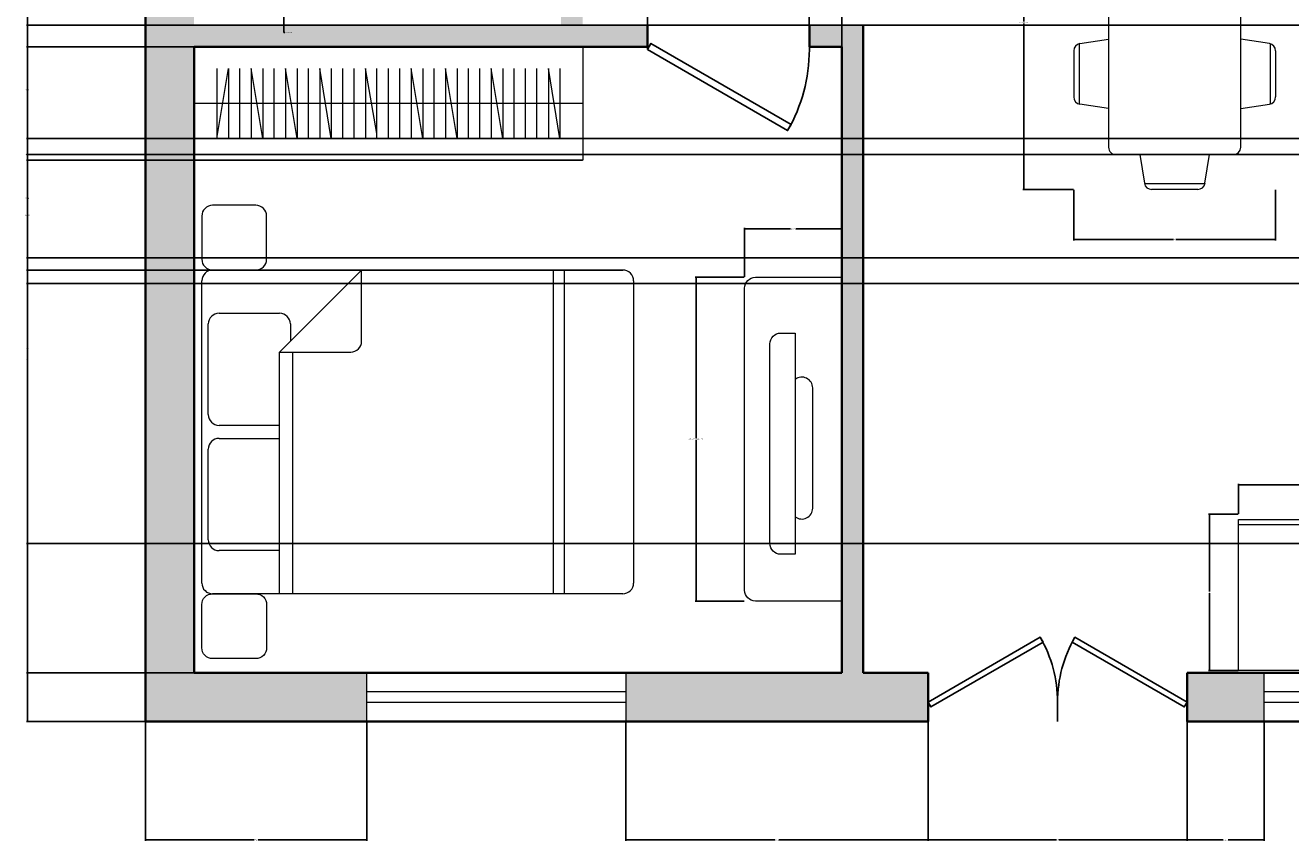
# Model space of a CAD drawing. Units: inches. Extents: x 2800 to 3283, y 1752 to 2114.
# Tile 1 of 6: x 2800 to 3035, y 1752 to 1903. Entities that reach past the tile are written whole.
import ezdxf

# ---------------------------------------------------------------- set-up
doc = ezdxf.new("R2010")
doc.units = ezdxf.units.IN
for name, color, linetype, lineweight in [('A-ANNO-DIMS', 2, 'Continuous', 18), ('A-DOOR', 3, 'Continuous', 25), ('A-EQPM', 8, 'Continuous', 18), ('A-FLOR-CASE', 8, 'Continuous', 18), ('A-FURN', 9, 'Continuous', 18), ('A-GLAZ', 4, 'Continuous', 18), ('A-WALL', 7, 'Continuous', 35)]:
    doc.layers.add(name, color=color, linetype=linetype, lineweight=lineweight)
doc.layers.add('A-WALL-PATT', color=18, linetype='Continuous', lineweight=13, true_color=0x000000)
doc.styles.get("Standard").update_dxf_attribs({"font": 'arial.ttf'})
doc.dimstyles.get("Standard").update_dxf_attribs({"dimtxt": 0.18, "dimasz": 0.18, "dimexe": 0.18, "dimexo": 0.0625, "dimgap": 0.09, "dimtad": 0, "dimtih": 1, "dimtoh": 1, "dimdec": 4, "dimzin": 0, "dimdsep": 46, "dimtxsty": 'Standard', "dimcen": 0.09, "dimadec": 0, "dimazin": 0, "dimtfac": 1, "dimtdec": 4, "dimtofl": 0, "dimtmove": 0, "dimatfit": 3, "dimfxl": 1, "dimtolj": 1, "dimtzin": 0, "dimarcsym": 0})

# ---------------------------------------------------------------- blocks, each defined once
blk = doc.blocks.new('Dining Set - 36 x 72 in.')
for p, q in [((-22.26, 25.81), (-23.48, 18)), ((-22.22, 26), (-5.78, 26)), ((-20.29, 27.5), (-7.71, 27.5)), ((-4.52, 18), (-5.74, 25.81)), ((5.74, 25.81), (4.52, 18)), ((5.78, 26), (22.22, 26)), ((7.71, 27.5), (20.29, 27.5)), ((23.48, 18), (22.26, 25.81)), ((34, 18), (-34, 18)), ((-36, 16), (-36, -16)), ((36, -16), (36, 16)), ((-44, 8.22), (-44, -8.22)), ((-43.81, 8.26), (-36, 9.48)), ((43.81, 8.26), (36, 9.48)), ((44, 8.22), (44, -8.22)), ((-45.5, 6.29), (-45.5, -6.29)), ((45.5, 6.29), (45.5, -6.29)), ((-36, -9.48), (-43.81, -8.26)), ((36, -9.48), (43.81, -8.26)), ((-34, -18), (34, -18)), ((-22.26, -25.81), (-23.48, -18)), ((-4.52, -18), (-5.74, -25.81)), ((5.74, -25.81), (4.52, -18)), ((23.48, -18), (22.26, -25.81)), ((-22.22, -26), (-5.78, -26)), ((-20.29, -27.5), (-7.71, -27.5)), ((5.78, -26), (22.22, -26)), ((7.71, -27.5), (20.29, -27.5))]:
    blk.add_line(p, q)
for centre, start, end in [((-20.29, 25.5), 90, 171.1198), ((-7.71, 25.5), 8.881, 90), ((7.71, 25.5), 90, 171.1198), ((20.29, 25.5), 8.881, 90), ((-34, 16), 90, 180), ((34, 16), 0, 90), ((-43.5, 6.29), 98.8806, 180), ((43.5, 6.29), 0, 81.1194), ((-43.5, -6.29), 180, 261.1194), ((43.5, -6.29), 278.8806, 0), ((-34, -16), 180, 270), ((34, -16), 270, 0), ((-20.29, -25.5), 188.8802, 270), ((-7.71, -25.5), 270, 351.1191), ((7.71, -25.5), 188.8802, 270), ((20.29, -25.5), 270, 351.1191)]:
    blk.add_arc(centre, 2, start, end)
blk = doc.blocks.new('Bed - Queen')
for p, q in [((2, 0), (58, 0)), ((0, -78), (0, -2)), ((10, -1.2), (26.8, -1.2)), ((33.2, -1.2), (50, -1.2)), ((60, -2), (60, -78)), ((8, -14.4), (8, -3.2)), ((28.8, -3.2), (28.8, -14.4)), ((31.2, -14.4), (31.2, -3.2)), ((52, -3.2), (52, -14.4)), ((0, -14.4), (44.8, -14.4)), ((60, -29.6), (44.8, -14.4)), ((44.8, -14.4), (44.8, -27.6)), ((50, -16.4), (46.8, -16.4)), ((44.8, -16.8), (0, -16.8)), ((46.8, -29.6), (60, -29.6)), ((0, -65.18), (60, -65.18)), ((0, -67.18), (60, -67.18)), ((58, -80), (2, -80))]:
    blk.add_line(p, q)
for centre, start, end in [((58, -2), 0, 90), ((2, -2), 90, 180), ((10, -3.2), 90, 180), ((26.8, -3.2), 0, 90), ((33.2, -3.2), 90, 180), ((50, -3.2), 0, 90), ((50, -14.4), 270, 0), ((46.8, -27.6), 180, 270), ((2, -78), 180, 270), ((58, -78), 270, 0)]:
    blk.add_arc(centre, 2, start, end)
blk = doc.blocks.new('Refrigerator-2 door - 36 in top')
for p, q in [((0, -26.999999), (36, -26.999999)), ((11, -27.999999), (11, -28.999999)), ((12, -26.999999), (12, -28.999999)), ((13, -28.999999), (13, -27.999999)), ((11, -28.999999), (13, -28.999999))]:
    blk.add_line(p, q)
blk.add_lwpolyline([(0, -27.999999), (0, 0), (36, 0), (36, -27.999999)], close=True)
blk = doc.blocks.new('*U12')
for p, q in [((0, 0), (0, -6)), ((40, 0), (40, -6))]:
    blk.add_line(p, q)
blk.add_lwpolyline([(0, 0), (34.64, 20), (35.52, 18.48), (0.87, -1.52)], close=True)
blk.add_arc((0, 0), 40, 0, 30)
blk = doc.blocks.new('*U13')
for p, q in [((0, 0), (0, 6)), ((40, 0), (40, 6))]:
    blk.add_line(p, q)
blk.add_lwpolyline([(0, 0), (34.64, -20), (35.52, -18.48), (0.87, 1.52)], close=True)
blk.add_arc((0, 0), 40, 330, 0)
blk = doc.blocks.new('WARDROBE-72')
for p, q in [((10.5, 72), (10.5, 0)), ((17, 63.53), (4, 63.53)), ((17, 61.41), (4, 61.41)), ((17, 59.29), (4, 59.29)), ((17, 52.94), (4, 52.94)), ((17, 50.82), (4, 50.82)), ((17, 44.47), (4, 44.47)), ((17, 38.12), (4, 38.12)), ((17, 36), (4, 36)), ((17, 33.88), (4, 33.88)), ((17, 29.65), (4, 29.65)), ((17, 27.53), (4, 27.53)), ((17, 21.18), (4, 21.18)), ((17, 14.82), (4, 14.82)), ((17, 8.47), (4, 8.47))]:
    blk.add_line(p, q)
for points in [[(0, 0), (0, 72), (21, 72), (21, 0), (0, 0), (21, 0)], [(4, 67.76), (17, 67.76), (4, 65.65), (17, 65.65)], [(4, 57.18), (17, 57.18), (4, 55.06), (17, 55.06)], [(4, 48.71), (17, 48.71), (4, 46.59), (17, 46.59)], [(4, 42.35), (17, 42.35), (4, 40.23), (17, 40.23)], [(16.02, 33.88), (4, 31.76), (17, 31.76)], [(4, 25.41), (17, 25.41), (4, 23.29), (17, 23.29)], [(4, 19.06), (17, 19.06), (4, 16.94), (17, 16.94)], [(4, 12.71), (17, 12.71), (4, 10.59), (17, 10.59)], [(4, 4.23), (17, 4.23), (4, 6.35), (17, 6.35)]]:
    blk.add_lwpolyline(points)
blk = doc.blocks.new('WIN-48')
for p, q in [((0, 5.5), (48, 5.5)), ((0, 3.5), (48, 3.5))]:
    blk.add_line(p, q)
for points in [[(0, 0), (0, 9)], [(48, 9), (48, 0)]]:
    blk.add_lwpolyline(points)
blk = doc.blocks.new('MEDIA-CONSOLE-60')
for points in [[(0, 60), (16, 60, -0.414214), (18, 58), (18, 2, -0.414214), (16, 0), (0, 0)], [(8.61, 51.33), (11.3, 51.33, -0.414214), (13.3, 49.33), (13.3, 12.33, -0.414214), (11.3, 10.33), (8.61, 10.33)]]:
    blk.add_lwpolyline(points, format="xyb", close=True)
blk.add_lwpolyline([(8.61, 15.1), (8.61, 47.68)])
blk.add_lwpolyline([(8.61, 44.37, 0.62446), (5.38, 42.79), (5.38, 20.5, 0.62446), (8.61, 18.92, 0.62446)], format="xyb")
blk = doc.blocks.new('NIGHTSTAND-12')
blk.add_lwpolyline([(2, 0), (10, 0, 0.414214), (12, 2), (12, 10, 0.414214), (10, 12), (2, 12, 0.414214), (0, 10), (0, 2, 0.414214)], format="xyb", close=True)
blk = doc.blocks.new('*D27')
at = {"layer": 'A-ANNO-DIMS', "color": 0, "lineweight": -2, "transparency": 16777216}
for p, q in [((2933.48, 1856.57), (2924.36, 1856.57)), ((2924.54, 1856.39), (2924.54, 1826.75)), ((2924.54, 1796.75), (2924.54, 1826.39)), ((2933.48, 1796.57), (2924.36, 1796.57))]:
    blk.add_line(p, q, dxfattribs=at)
at = {"layer": 'A-ANNO-DIMS', "color": 0, "transparency": 16777216}
for points in [[(2924.51, 1856.39), (2924.57, 1856.39), (2924.54, 1856.57)], [(2924.51, 1796.75), (2924.57, 1796.75), (2924.54, 1796.57)]]:
    blk.add_solid(points, dxfattribs=at)
at = {"layer": 'Defpoints', "color": 0, "transparency": 16777216}
for p in [(2933.54, 1856.57), (2924.54, 1796.57), (2933.54, 1796.57)]:
    blk.add_point(p, dxfattribs=at)
at = {"layer": 'A-ANNO-DIMS', "color": 0, "transparency": 16777216, "insert": (2924.54, 1826.57), "char_height": 0.18, "attachment_point": 5}
blk.add_mtext('\\A1;MEDIA CONSOLE 60 TYP.', dxfattribs=at)
blk = doc.blocks.new('*D28')
at = {"layer": 'A-ANNO-DIMS', "color": 0, "lineweight": -2, "transparency": 16777216}
for p, q in [((2933.54, 1856.63), (2933.54, 1865.75)), ((2933.72, 1865.57), (2942.02, 1865.57)), ((2951.36, 1865.57), (2943.06, 1865.57)), ((2951.54, 1856.63), (2951.54, 1865.75))]:
    blk.add_line(p, q, dxfattribs=at)
at = {"layer": 'A-ANNO-DIMS', "color": 0, "transparency": 16777216}
for points in [[(2933.72, 1865.6), (2933.72, 1865.54), (2933.54, 1865.57)], [(2951.36, 1865.6), (2951.36, 1865.54), (2951.54, 1865.57)]]:
    blk.add_solid(points, dxfattribs=at)
at = {"layer": 'Defpoints', "color": 0, "transparency": 16777216}
for p in [(2933.54, 1865.57), (2933.54, 1856.57), (2951.54, 1856.57)]:
    blk.add_point(p, dxfattribs=at)
at = {"layer": 'A-ANNO-DIMS', "color": 0, "transparency": 16777216, "insert": (2942.54, 1865.57), "char_height": 0.18, "attachment_point": 5}
blk.add_mtext('\\A1;18 TYP.', dxfattribs=at)
blk = doc.blocks.new('*D35')
at = {"layer": 'A-ANNO-DIMS', "color": 0, "lineweight": -2, "transparency": 16777216}
for p, q in [((2994.48, 1934.72), (2985.08, 1934.72)), ((2985.26, 1934.54), (2985.26, 1903.97)), ((2985.26, 1873.03), (2985.26, 1903.6)), ((2994.48, 1872.85), (2985.08, 1872.85))]:
    blk.add_line(p, q, dxfattribs=at)
at = {"layer": 'A-ANNO-DIMS', "color": 0, "transparency": 16777216}
for points in [[(2985.23, 1934.54), (2985.29, 1934.54), (2985.26, 1934.72)], [(2985.23, 1873.03), (2985.29, 1873.03), (2985.26, 1872.85)]]:
    blk.add_solid(points, dxfattribs=at)
at = {"layer": 'Defpoints', "color": 0, "transparency": 16777216}
for p in [(2994.54, 1934.72), (2985.26, 1872.85), (2994.54, 1872.85)]:
    blk.add_point(p, dxfattribs=at)
at = {"layer": 'A-ANNO-DIMS', "color": 0, "transparency": 16777216, "insert": (2985.26, 1903.79), "char_height": 0.18, "attachment_point": 5}
blk.add_mtext('\\A1;DINING SET 62', dxfattribs=at)
blk = doc.blocks.new('*D36')
at = {"layer": 'A-ANNO-DIMS', "color": 0, "lineweight": -2, "transparency": 16777216}
for p, q in [((2994.54, 1872.79), (2994.54, 1863.39)), ((3031.94, 1872.79), (3031.94, 1863.39)), ((2994.72, 1863.57), (3013.02, 1863.57)), ((3031.76, 1863.57), (3013.46, 1863.57))]:
    blk.add_line(p, q, dxfattribs=at)
at = {"layer": 'A-ANNO-DIMS', "color": 0, "transparency": 16777216}
for points in [[(2994.72, 1863.6), (2994.72, 1863.54), (2994.54, 1863.57)], [(3031.76, 1863.6), (3031.76, 1863.54), (3031.94, 1863.57)]]:
    blk.add_solid(points, dxfattribs=at)
at = {"layer": 'Defpoints', "color": 0, "transparency": 16777216}
for p in [(2994.54, 1872.85), (3031.94, 1872.85), (3031.94, 1863.57)]:
    blk.add_point(p, dxfattribs=at)
at = {"layer": 'A-ANNO-DIMS', "color": 0, "transparency": 16777216, "insert": (3013.24, 1863.57), "char_height": 0.18, "attachment_point": 5}
blk.add_mtext('\\A1;37', dxfattribs=at)
blk = doc.blocks.new('*D41')
at = {"layer": 'A-ANNO-DIMS', "color": 0, "lineweight": -2, "transparency": 16777216}
for p, q in [((3025.08, 1812.76), (3025.08, 1818.28)), ((3025.26, 1818.1), (3041.83, 1818.1)), ((3060.9, 1818.1), (3044.33, 1818.1)), ((3061.08, 1812.76), (3061.08, 1818.28))]:
    blk.add_line(p, q, dxfattribs=at)
at = {"layer": 'A-ANNO-DIMS', "color": 0, "transparency": 16777216}
for points in [[(3025.26, 1818.13), (3025.26, 1818.07), (3025.08, 1818.1)], [(3060.9, 1818.13), (3060.9, 1818.07), (3061.08, 1818.1)]]:
    blk.add_solid(points, dxfattribs=at)
at = {"layer": 'Defpoints', "color": 0, "transparency": 16777216}
for p in [(3025.08, 1818.1), (3025.08, 1812.7), (3061.08, 1812.7)]:
    blk.add_point(p, dxfattribs=at)
at = {"layer": 'A-ANNO-DIMS', "color": 0, "transparency": 16777216, "insert": (3043.08, 1818.1), "char_height": 0.18, "attachment_point": 5}
blk.add_mtext('\\A1;REFRIGERATOR 36', dxfattribs=at)
blk = doc.blocks.new('*D42')
at = {"layer": 'A-ANNO-DIMS', "color": 0, "lineweight": -2, "transparency": 16777216}
for p, q in [((3025.02, 1812.7), (3019.5, 1812.7)), ((3019.68, 1812.52), (3019.68, 1798.38)), ((3019.68, 1783.88), (3019.68, 1798.02)), ((3025.02, 1783.7), (3019.5, 1783.7))]:
    blk.add_line(p, q, dxfattribs=at)
at = {"layer": 'A-ANNO-DIMS', "color": 0, "transparency": 16777216}
for points in [[(3019.65, 1812.52), (3019.71, 1812.52), (3019.68, 1812.7)], [(3019.65, 1783.88), (3019.71, 1783.88), (3019.68, 1783.7)]]:
    blk.add_solid(points, dxfattribs=at)
at = {"layer": 'Defpoints', "color": 0, "transparency": 16777216}
for p in [(3025.08, 1812.7), (3019.68, 1783.7), (3025.08, 1783.7)]:
    blk.add_point(p, dxfattribs=at)
at = {"layer": 'A-ANNO-DIMS', "color": 0, "transparency": 16777216, "insert": (3019.68, 1798.2), "char_height": 0.18, "attachment_point": 5}
blk.add_mtext('\\A1;29', dxfattribs=at)
blk = doc.blocks.new('*D44')
at = {"layer": 'A-ANNO-DIMS', "color": 0, "lineweight": -2, "transparency": 16777216}
for p, q in [((2822.48, 2092.27), (2800.45, 2092.27)), ((2800.63, 2092.09), (2800.63, 1933.45)), ((2800.63, 1774.45), (2800.63, 1933.09)), ((2822.48, 1774.27), (2800.45, 1774.27))]:
    blk.add_line(p, q, dxfattribs=at)
at = {"layer": 'A-ANNO-DIMS', "color": 0, "transparency": 16777216}
for points in [[(2800.6, 2092.09), (2800.66, 2092.09), (2800.63, 2092.27)], [(2800.6, 1774.45), (2800.66, 1774.45), (2800.63, 1774.27)]]:
    blk.add_solid(points, dxfattribs=at)
at = {"layer": 'Defpoints', "color": 0, "transparency": 16777216}
for p in [(2800.63, 2092.27), (2822.54, 2092.27), (2822.54, 1774.27)]:
    blk.add_point(p, dxfattribs=at)
at = {"layer": 'A-ANNO-DIMS', "color": 0, "transparency": 16777216, "insert": (2800.63, 1933.27), "char_height": 0.18, "attachment_point": 5}
blk.add_mtext('\\A1;318', dxfattribs=at)
blk = doc.blocks.new('*D51')
at = {"layer": 'A-ANNO-DIMS', "color": 0, "lineweight": -2, "transparency": 16777216}
for p, q in [((2831.48, 1899.27), (2800.45, 1899.27)), ((2800.63, 1899.09), (2800.63, 1841.45)), ((2800.63, 1783.45), (2800.63, 1841.09)), ((2831.48, 1783.27), (2800.45, 1783.27))]:
    blk.add_line(p, q, dxfattribs=at)
at = {"layer": 'A-ANNO-DIMS', "color": 0, "transparency": 16777216}
for points in [[(2800.6, 1899.09), (2800.66, 1899.09), (2800.63, 1899.27)], [(2800.6, 1783.45), (2800.66, 1783.45), (2800.63, 1783.27)]]:
    blk.add_solid(points, dxfattribs=at)
at = {"layer": 'Defpoints', "color": 0, "transparency": 16777216}
for p in [(2800.63, 1899.27), (2831.54, 1899.27), (2831.54, 1783.27)]:
    blk.add_point(p, dxfattribs=at)
at = {"layer": 'A-ANNO-DIMS', "color": 0, "transparency": 16777216, "insert": (2800.63, 1841.27), "char_height": 0.18, "attachment_point": 5}
blk.add_mtext('\\A1;116', dxfattribs=at)
blk = doc.blocks.new('*D59')
at = {"layer": 'A-ANNO-DIMS', "color": 0, "lineweight": -2, "transparency": 16777216}
for p, q in [((2822.54, 1774.21), (2822.54, 1752.17)), ((2863.53, 1774.21), (2863.53, 1752.17)), ((2822.72, 1752.35), (2842.64, 1752.35)), ((2863.35, 1752.35), (2843.43, 1752.35))]:
    blk.add_line(p, q, dxfattribs=at)
at = {"layer": 'A-ANNO-DIMS', "color": 0, "transparency": 16777216}
for points in [[(2822.72, 1752.38), (2822.72, 1752.32), (2822.54, 1752.35)], [(2863.35, 1752.38), (2863.35, 1752.32), (2863.53, 1752.35)]]:
    blk.add_solid(points, dxfattribs=at)
at = {"layer": 'Defpoints', "color": 0, "transparency": 16777216}
for p in [(2822.54, 1774.27), (2863.53, 1774.27), (2863.53, 1752.35)]:
    blk.add_point(p, dxfattribs=at)
at = {"layer": 'A-ANNO-DIMS', "color": 0, "transparency": 16777216, "insert": (2843.04, 1752.35), "char_height": 0.18, "attachment_point": 5}
blk.add_mtext('\\A1;40.99', dxfattribs=at)
blk = doc.blocks.new('*D60')
at = {"layer": 'A-ANNO-DIMS', "color": 0, "lineweight": -2, "transparency": 16777216}
for p, q in [((2911.53, 1774.21), (2911.53, 1752.17)), ((2967.54, 1774.21), (2967.54, 1752.17)), ((2911.71, 1752.35), (2939.16, 1752.35)), ((2967.36, 1752.35), (2939.91, 1752.35))]:
    blk.add_line(p, q, dxfattribs=at)
at = {"layer": 'A-ANNO-DIMS', "color": 0, "transparency": 16777216}
for points in [[(2911.71, 1752.38), (2911.71, 1752.32), (2911.53, 1752.35)], [(2967.36, 1752.38), (2967.36, 1752.32), (2967.54, 1752.35)]]:
    blk.add_solid(points, dxfattribs=at)
at = {"layer": 'Defpoints', "color": 0, "transparency": 16777216}
for p in [(2911.53, 1774.27), (2967.54, 1774.27), (2967.54, 1752.35)]:
    blk.add_point(p, dxfattribs=at)
at = {"layer": 'A-ANNO-DIMS', "color": 0, "transparency": 16777216, "insert": (2939.54, 1752.35), "char_height": 0.18, "attachment_point": 5}
blk.add_mtext('\\A1;56.01', dxfattribs=at)
blk = doc.blocks.new('*D61')
at = {"layer": 'A-ANNO-DIMS', "color": 0, "lineweight": -2, "transparency": 16777216}
for p, q in [((2967.54, 1774.21), (2967.54, 1752.17)), ((3015.54, 1774.21), (3015.54, 1752.17)), ((2967.72, 1752.35), (2991.32, 1752.35)), ((3015.36, 1752.35), (2991.77, 1752.35))]:
    blk.add_line(p, q, dxfattribs=at)
at = {"layer": 'A-ANNO-DIMS', "color": 0, "transparency": 16777216}
for points in [[(2967.72, 1752.38), (2967.72, 1752.32), (2967.54, 1752.35)], [(3015.36, 1752.38), (3015.36, 1752.32), (3015.54, 1752.35)]]:
    blk.add_solid(points, dxfattribs=at)
at = {"layer": 'Defpoints', "color": 0, "transparency": 16777216}
for p in [(2967.54, 1774.27), (3015.54, 1774.27), (3015.54, 1752.35)]:
    blk.add_point(p, dxfattribs=at)
at = {"layer": 'A-ANNO-DIMS', "color": 0, "transparency": 16777216, "insert": (2991.54, 1752.35), "char_height": 0.18, "attachment_point": 5}
blk.add_mtext('\\A1;48', dxfattribs=at)
blk = doc.blocks.new('*D62')
at = {"layer": 'A-ANNO-DIMS', "color": 0, "lineweight": -2, "transparency": 16777216}
for p, q in [((3015.54, 1774.21), (3015.54, 1752.17)), ((3029.8, 1774.21), (3029.8, 1752.17)), ((3015.72, 1752.35), (3022.22, 1752.35)), ((3029.62, 1752.35), (3023.13, 1752.35))]:
    blk.add_line(p, q, dxfattribs=at)
at = {"layer": 'A-ANNO-DIMS', "color": 0, "transparency": 16777216}
for points in [[(3015.72, 1752.38), (3015.72, 1752.32), (3015.54, 1752.35)], [(3029.62, 1752.38), (3029.62, 1752.32), (3029.8, 1752.35)]]:
    blk.add_solid(points, dxfattribs=at)
at = {"layer": 'Defpoints', "color": 0, "transparency": 16777216}
for p in [(3015.54, 1774.27), (3029.8, 1774.27), (3029.8, 1752.35)]:
    blk.add_point(p, dxfattribs=at)
at = {"layer": 'A-ANNO-DIMS', "color": 0, "transparency": 16777216, "insert": (3022.67, 1752.35), "char_height": 0.18, "attachment_point": 5}
blk.add_mtext('\\A1;14.258', dxfattribs=at)
blk = doc.blocks.new('*D66')
at = {"layer": 'A-ANNO-DIMS', "color": 0, "lineweight": -2, "transparency": 16777216}
for p, q in [((2915.54, 1899.33), (2915.54, 2114.36)), ((2915.72, 2114.18), (2930.32, 2114.18)), ((2945.36, 2114.18), (2930.76, 2114.18)), ((2945.54, 1899.33), (2945.54, 2114.36))]:
    blk.add_line(p, q, dxfattribs=at)
at = {"layer": 'A-ANNO-DIMS', "color": 0, "transparency": 16777216}
for points in [[(2915.72, 2114.21), (2915.72, 2114.15), (2915.54, 2114.18)], [(2945.36, 2114.21), (2945.36, 2114.15), (2945.54, 2114.18)]]:
    blk.add_solid(points, dxfattribs=at)
at = {"layer": 'Defpoints', "color": 0, "transparency": 16777216}
for p in [(2945.54, 2114.18), (2915.54, 1899.27), (2945.54, 1899.27)]:
    blk.add_point(p, dxfattribs=at)
at = {"layer": 'A-ANNO-DIMS', "color": 0, "transparency": 16777216, "insert": (2930.54, 2114.18), "char_height": 0.18, "attachment_point": 5}
blk.add_mtext('\\A1;30', dxfattribs=at)
blk = doc.blocks.new('*D67')
at = {"layer": 'A-ANNO-DIMS', "color": 0, "lineweight": -2, "transparency": 16777216}
for p, q in [((2945.54, 1899.33), (2945.54, 2114.36)), ((2945.72, 2114.18), (2948.39, 2114.18)), ((2951.36, 2114.18), (2948.69, 2114.18)), ((2951.54, 1899.33), (2951.54, 2114.36))]:
    blk.add_line(p, q, dxfattribs=at)
at = {"layer": 'A-ANNO-DIMS', "color": 0, "transparency": 16777216}
for points in [[(2945.72, 2114.21), (2945.72, 2114.15), (2945.54, 2114.18)], [(2951.36, 2114.21), (2951.36, 2114.15), (2951.54, 2114.18)]]:
    blk.add_solid(points, dxfattribs=at)
at = {"layer": 'Defpoints', "color": 0, "transparency": 16777216}
for p in [(2951.54, 2114.18), (2945.54, 1899.27), (2951.54, 1899.27)]:
    blk.add_point(p, dxfattribs=at)
at = {"layer": 'A-ANNO-DIMS', "color": 0, "transparency": 16777216, "insert": (2948.54, 2114.18), "char_height": 0.18, "attachment_point": 5}
blk.add_mtext('\\A1;6', dxfattribs=at)
blk = doc.blocks.new('*D71')
at = {"layer": 'A-ANNO-DIMS', "color": 0, "lineweight": -2, "transparency": 16777216}
for p, q in [((3037.48, 1903.27), (2800.45, 1903.27)), ((2800.63, 1903.09), (2800.63, 1879.54)), ((2800.63, 1855.63), (2800.63, 1879.18)), ((3037.48, 1855.45), (2800.45, 1855.45))]:
    blk.add_line(p, q, dxfattribs=at)
at = {"layer": 'A-ANNO-DIMS', "color": 0, "transparency": 16777216}
for points in [[(2800.6, 1903.09), (2800.66, 1903.09), (2800.63, 1903.27)], [(2800.6, 1855.63), (2800.66, 1855.63), (2800.63, 1855.45)]]:
    blk.add_solid(points, dxfattribs=at)
at = {"layer": 'Defpoints', "color": 0, "transparency": 16777216}
for p in [(2800.63, 1903.27), (3037.54, 1903.27), (3037.54, 1855.45)]:
    blk.add_point(p, dxfattribs=at)
at = {"layer": 'A-ANNO-DIMS', "color": 0, "transparency": 16777216, "insert": (2800.63, 1879.36), "char_height": 0.18, "attachment_point": 5}
blk.add_mtext('\\A1;47.82', dxfattribs=at)
blk = doc.blocks.new('*D73')
at = {"layer": 'A-ANNO-DIMS', "color": 0, "lineweight": -2, "transparency": 16777216}
for p, q in [((3103.48, 1879.34), (2800.45, 1879.34)), ((2800.63, 1879.16), (2800.63, 1843.49)), ((2800.63, 1807.45), (2800.63, 1843.12)), ((3103.48, 1807.27), (2800.45, 1807.27))]:
    blk.add_line(p, q, dxfattribs=at)
at = {"layer": 'A-ANNO-DIMS', "color": 0, "transparency": 16777216}
for points in [[(2800.6, 1879.16), (2800.66, 1879.16), (2800.63, 1879.34)], [(2800.6, 1807.45), (2800.66, 1807.45), (2800.63, 1807.27)]]:
    blk.add_solid(points, dxfattribs=at)
at = {"layer": 'Defpoints', "color": 0, "transparency": 16777216}
for p in [(2800.63, 1879.34), (3103.54, 1879.34), (3103.54, 1807.27)]:
    blk.add_point(p, dxfattribs=at)
at = {"layer": 'A-ANNO-DIMS', "color": 0, "transparency": 16777216, "insert": (2800.63, 1843.31), "char_height": 0.18, "attachment_point": 5}
blk.add_mtext('\\A1;72.07', dxfattribs=at)
blk = doc.blocks.new('*D76')
at = {"layer": 'A-ANNO-DIMS', "color": 0, "lineweight": -2, "transparency": 16777216}
for p, q in [((3095.48, 1903.27), (2800.45, 1903.27)), ((2800.63, 1903.09), (2800.63, 1891.49)), ((2800.63, 1879.52), (2800.63, 1891.12)), ((3103.48, 1879.34), (2800.45, 1879.34))]:
    blk.add_line(p, q, dxfattribs=at)
at = {"layer": 'A-ANNO-DIMS', "color": 0, "transparency": 16777216}
for points in [[(2800.6, 1903.09), (2800.66, 1903.09), (2800.63, 1903.27)], [(2800.6, 1879.52), (2800.66, 1879.52), (2800.63, 1879.34)]]:
    blk.add_solid(points, dxfattribs=at)
at = {"layer": 'Defpoints', "color": 0, "transparency": 16777216}
for p in [(3095.54, 1903.27), (2800.63, 1879.34), (3103.54, 1879.34)]:
    blk.add_point(p, dxfattribs=at)
at = {"layer": 'A-ANNO-DIMS', "color": 0, "transparency": 16777216, "insert": (2800.63, 1891.31), "char_height": 0.18, "attachment_point": 5}
blk.add_mtext('\\A1;23.93', dxfattribs=at)
blk = doc.blocks.new('*D83')
at = {"layer": 'A-ANNO-DIMS', "color": 0, "lineweight": -2, "transparency": 16777216}
for p, q in [((2903.48, 1878.27), (2800.45, 1878.27)), ((2800.63, 1878.09), (2800.63, 1868.28)), ((2800.63, 1858.1), (2800.63, 1867.91)), ((2910.9, 1857.92), (2800.45, 1857.92))]:
    blk.add_line(p, q, dxfattribs=at)
at = {"layer": 'A-ANNO-DIMS', "color": 0, "transparency": 16777216}
for points in [[(2800.6, 1878.09), (2800.66, 1878.09), (2800.63, 1878.27)], [(2800.6, 1858.1), (2800.66, 1858.1), (2800.63, 1857.92)]]:
    blk.add_solid(points, dxfattribs=at)
at = {"layer": 'Defpoints', "color": 0, "transparency": 16777216}
for p in [(2903.54, 1878.27), (2800.63, 1857.92), (2910.97, 1857.92)]:
    blk.add_point(p, dxfattribs=at)
at = {"layer": 'A-ANNO-DIMS', "color": 0, "transparency": 16777216, "insert": (2800.63, 1868.1), "char_height": 0.18, "attachment_point": 5}
blk.add_mtext('\\A1;20.348', dxfattribs=at)
blk = doc.blocks.new('*D84')
at = {"layer": 'A-ANNO-DIMS', "color": 0, "lineweight": -2, "transparency": 16777216}
for p, q in [((3179.48, 1882.27), (2800.45, 1882.27)), ((2800.63, 1882.09), (2800.63, 1871.42)), ((2800.63, 1860.39), (2800.63, 1871.06)), ((3172.07, 1860.21), (2800.45, 1860.21))]:
    blk.add_line(p, q, dxfattribs=at)
at = {"layer": 'A-ANNO-DIMS', "color": 0, "transparency": 16777216}
for points in [[(2800.6, 1882.09), (2800.66, 1882.09), (2800.63, 1882.27)], [(2800.6, 1860.39), (2800.66, 1860.39), (2800.63, 1860.21)]]:
    blk.add_solid(points, dxfattribs=at)
at = {"layer": 'Defpoints', "color": 0, "transparency": 16777216}
for p in [(3179.54, 1882.27), (2800.63, 1860.21), (3172.14, 1860.21)]:
    blk.add_point(p, dxfattribs=at)
at = {"layer": 'A-ANNO-DIMS', "color": 0, "transparency": 16777216, "insert": (2800.63, 1871.24), "char_height": 0.18, "attachment_point": 5}
blk.add_mtext('\\A1;22.06', dxfattribs=at)
blk = doc.blocks.new('*D87')
at = {"layer": 'A-ANNO-DIMS', "color": 0, "lineweight": -2, "transparency": 16777216}
for p, q in [((2848.06, 1921.79), (2848.24, 1921.79)), ((2848.15, 1921.7), (2848.15, 1921.88)), ((2848.15, 1901.96), (2848.15, 1909.22)), ((2848.33, 1901.96), (2848.15, 1901.96))]:
    blk.add_line(p, q, dxfattribs=at)
at = {"layer": 'A-ANNO-DIMS', "color": 0, "transparency": 16777216}
blk.add_solid([(2848.18, 1909.22), (2848.12, 1909.22), (2848.15, 1909.4)], dxfattribs=at)
at = {"layer": 'Defpoints', "color": 0, "transparency": 16777216}
for p in [(2848.15, 1921.79), (2848.15, 1909.4)]:
    blk.add_point(p, dxfattribs=at)
at = {"layer": 'A-ANNO-DIMS', "color": 0, "transparency": 16777216, "insert": (2849.06, 1901.96), "char_height": 0.18, "attachment_point": 5}
blk.add_mtext('\\A1;2X R12.391', dxfattribs=at)

msp = doc.modelspace()

# ---------------------------------------------------------------- hatches: boundary and pattern name
at = {"layer": 'A-WALL-PATT'}
h = msp.add_hatch(color=256, dxfattribs=at)
h.dxf.hatch_style = 1
h.paths.add_polyline_path([(2863.5307, 1783.2695), (2831.5432, 1783.2695), (2831.5432, 1899.2695), (2903.5432, 1899.2695), (2915.5432, 1899.2695), (2915.5432, 1903.2695), (2903.5432, 1903.2695), (2903.5432, 1933.2695), (2899.5432, 1933.2695), (2899.5432, 1903.2695), (2831.5432, 1903.2695), (2831.5432, 1922.3547), (2822.5432, 1922.3547), (2822.5432, 1774.2695), (2863.5307, 1774.2695)])
h = msp.add_hatch(color=256, dxfattribs=at)
h.dxf.hatch_style = 1
h.paths.add_polyline_path([(2967.5432, 1783.2695), (2955.5432, 1783.2695), (2955.5432, 1903.2695), (2945.5432, 1903.2695), (2945.5432, 1899.2695), (2951.5432, 1899.2695), (2951.5432, 1783.2695), (2911.5307, 1783.2695), (2911.5307, 1774.2695), (2967.5432, 1774.2695)])
h = msp.add_hatch(color=256, dxfattribs=at)
h.dxf.hatch_style = 1
h.paths.add_polyline_path([(3029.8011, 1783.2695), (3015.5432, 1783.2695), (3015.5432, 1774.2695), (3029.8011, 1774.2695)])

# ---------------------------------------------------------------- linework, layer by layer
at = {"layer": 'A-WALL'}
for p, q in [((2915.5432, 1899.2695), (2915.5432, 1903.2695)), ((2945.5432, 1899.2695), (2945.5432, 1903.2695)), ((2955.5432, 1783.2695), (2955.5432, 1903.2695)), ((2831.5432, 1783.2695), (2831.5432, 1899.2695)), ((2915.5432, 1899.2695), (2831.5432, 1899.2695)), ((2951.5432, 1899.2695), (2945.5432, 1899.2695)), ((2951.5432, 1783.2695), (2951.5432, 1899.2695)), ((2951.5432, 1783.2695), (2831.5432, 1783.2695)), ((2967.5432, 1783.2695), (2955.5432, 1783.2695)), ((2967.5432, 1783.2695), (2967.5432, 1774.2695)), ((3127.5432, 1783.2695), (3015.5432, 1783.2695)), ((3015.5432, 1783.2695), (3015.5432, 1774.2695))]:
    msp.add_line(p, q, dxfattribs=at)
msp.add_lwpolyline([(2967.5432, 1774.2695), (2822.5432, 1774.2695), (2822.5432, 2092.2695), (3260.5432, 2092.2695), (3260.5432, 1774.2695), (3015.5432, 1774.2695)], dxfattribs=at)

# ---------------------------------------------------------------- block references
at = {"layer": 'A-DOOR'}
for name, p, xscale, yscale, zscale in [('*U13', (2915.5432, 1898.7695), 0.75, 0.75, 0.75), ('*U12', (2967.5432, 1777.8695), 0.6, 0.6, 0.6), ('*U12', (3015.5432, 1777.8695), -0.6, 0.6, 0.6)]:
    msp.add_blockref(name, p, dxfattribs=dict(at, xscale=xscale, yscale=yscale, zscale=zscale))
at = {"layer": 'A-EQPM', "rotation": 180}
msp.add_blockref('Refrigerator-2 door - 36 in top', (3061.0792, 1783.7005), dxfattribs=at)
at = {"layer": 'A-FLOR-CASE', "rotation": 270}
msp.add_blockref('WARDROBE-72', (2831.5437, 1899.2697), dxfattribs=at)
at = {"layer": 'A-FURN', "xscale": 0.6798973634336658, "yscale": 0.6798973634336658, "zscale": 0.6798973634336658, "rotation": 270}
msp.add_blockref('Dining Set - 36 x 72 in.', (3013.2412, 1903.787), dxfattribs=at)
at = {"layer": 'A-FURN'}
msp.add_blockref('NIGHTSTAND-12', (2832.967, 1857.922), dxfattribs=at)
for name, p, rotation in [('Bed - Queen', (2832.9674, 1797.9218), 89.99999999999999), ('MEDIA-CONSOLE-60', (2951.5433, 1856.5689), 180)]:
    msp.add_blockref(name, p, dxfattribs=dict(at, rotation=rotation))
at = {"layer": 'A-FURN', "extrusion": (0, 0, -1), "zscale": -1, "rotation": 180}
msp.add_blockref('NIGHTSTAND-12', (-2832.967, 1797.9216), dxfattribs=at)
at = {"layer": 'A-GLAZ', "rotation": 180}
for p in [(2911.5306, 1783.269), (3077.801, 1783.269)]:
    msp.add_blockref('WIN-48', p, dxfattribs=at)

# ---------------------------------------------------------------- dimensions: what is measured, and where the dimension line sits
at = {"layer": 'A-ANNO-DIMS'}
for base, p1, p2, override, picture, middle in [((2945.5432, 2114.1845), (2915.5432, 1899.2695), (2945.5432, 1899.2695), {"dimdec": 0, "dimlfac": 1, "dimrnd": 0, "dimzin": 0, "dimdsep": 46, "dimlunit": 2}, '*D66', (2930.5432, 2114.1845)), ((2951.5432, 2114.1845), (2945.5432, 1899.2695), (2951.5432, 1899.2695), {"dimdec": 0, "dimlfac": 1, "dimrnd": 0, "dimzin": 0, "dimdsep": 46, "dimlunit": 2}, '*D67', (2948.5432, 2114.1845)), ((3031.9384, 1863.5711), (2994.5441, 1872.8517), (3031.9384, 1872.8517), {"dimdec": 0, "dimlfac": 1, "dimrnd": 0, "dimzin": 0, "dimdsep": 46, "dimlunit": 2}, '*D36', (3013.2412, 1863.5711)), ((2863.5307, 1752.3545), (2822.5432, 1774.2695), (2863.5307, 1774.2695), {"dimdec": 2, "dimlfac": 1, "dimrnd": 0, "dimzin": 0, "dimdsep": 46, "dimlunit": 2}, '*D59', (2843.037, 1752.3545)), ((2967.5432, 1752.3545), (2911.5307, 1774.2695), (2967.5432, 1774.2695), {"dimdec": 2, "dimlfac": 1, "dimrnd": 0, "dimzin": 0, "dimdsep": 46, "dimlunit": 2}, '*D60', (2939.537, 1752.3545)), ((3015.5432, 1752.3545), (2967.5432, 1774.2695), (3015.5432, 1774.2695), {"dimdec": 0, "dimlfac": 1, "dimrnd": 0, "dimzin": 0, "dimdsep": 46, "dimlunit": 2}, '*D61', (2991.5432, 1752.3545)), ((3029.8011, 1752.3545), (3015.5432, 1774.2695), (3029.8011, 1774.2695), {"dimdec": 3, "dimlfac": 1, "dimrnd": 0, "dimzin": 0, "dimdsep": 46, "dimlunit": 2}, '*D62', (3022.6722, 1752.3545))]:
    dim = msp.add_linear_dim(base=base, p1=p1, p2=p2, dimstyle='Standard', override=override, dxfattribs=at)
    dim.commit()
    dim.dimension.update_dxf_attribs({"geometry": picture, "text_midpoint": middle})
for base, p1, p2, angle, override, picture, middle in [((2800.6282, 2092.2695), (2822.5432, 1774.2695), (2822.5432, 2092.2695), 90, {"dimdec": 0, "dimlfac": 1, "dimrnd": 0, "dimzin": 0, "dimdsep": 46, "dimlunit": 2}, '*D44', (2800.6282, 1933.2695)), ((2800.6282, 1903.2695), (3037.5432, 1855.4517), (3037.5432, 1903.2695), 90, {"dimdec": 2, "dimlfac": 1, "dimrnd": 0, "dimzin": 0, "dimdsep": 46, "dimlunit": 2}, '*D71', (2800.6282, 1879.3606)), ((2800.6282, 1879.3408), (3095.5432, 1903.2695), (3103.5432, 1879.3408), 90, {"dimdec": 2, "dimlfac": 1, "dimrnd": 0, "dimzin": 0, "dimdsep": 46, "dimlunit": 2}, '*D76', (2800.6282, 1891.3052)), ((2800.6282, 1899.2695), (2831.5432, 1783.2695), (2831.5432, 1899.2695), 90, {"dimdec": 0, "dimlfac": 1, "dimrnd": 0, "dimzin": 0, "dimdsep": 46, "dimlunit": 2}, '*D51', (2800.6282, 1841.2695)), ((2800.6282, 1860.2087), (3179.5432, 1882.2695), (3172.1372, 1860.2087), 90, {"dimdec": 2, "dimlfac": 1, "dimrnd": 0, "dimzin": 0, "dimdsep": 46, "dimlunit": 2}, '*D84', (2800.6282, 1871.2391)), ((2800.6282, 1857.9218), (2903.5432, 1878.2695), (2910.9675, 1857.9218), 90, {"dimdec": 3, "dimlfac": 1, "dimrnd": 0, "dimzin": 0, "dimdsep": 46, "dimlunit": 2}, '*D83', (2800.6282, 1868.0956)), ((2800.6282, 1879.3408), (3103.5432, 1807.2695), (3103.5432, 1879.3408), 90, {"dimdec": 2, "dimlfac": 1, "dimrnd": 0, "dimzin": 0, "dimdsep": 46, "dimlunit": 2}, '*D73', (2800.6282, 1843.3052)), ((3019.6792, 1783.7005), (3025.0792, 1812.7005), (3025.0792, 1783.7005), 270, {"dimdec": 0, "dimlfac": 1, "dimrnd": 0, "dimzin": 0, "dimdsep": 46, "dimlunit": 2}, '*D42', (3019.6792, 1798.2005))]:
    dim = msp.add_linear_dim(base=base, p1=p1, p2=p2, angle=angle, dimstyle='Standard', override=override, dxfattribs=at)
    dim.commit()
    dim.dimension.update_dxf_attribs({"geometry": picture, "text_midpoint": middle})
for base, p1, p2, angle, text, picture, middle in [((2985.2635, 1872.8517), (2994.5441, 1934.7224), (2994.5441, 1872.8517), 270, 'DINING SET <>', '*D35', (2985.2635, 1903.787)), ((2933.5432, 1865.5693), (2951.5432, 1856.5693), (2933.5432, 1856.5693), 180, '<> TYP.', '*D28', (2942.5432, 1865.5693)), ((2924.5432, 1796.5693), (2933.5432, 1856.5693), (2933.5432, 1796.5693), 270, 'MEDIA CONSOLE <> TYP.', '*D27', (2924.5432, 1826.5693)), ((3025.0792, 1818.1005), (3061.0792, 1812.7005), (3025.0792, 1812.7005), 180, 'REFRIGERATOR <>', '*D41', (3043.0792, 1818.1005))]:
    dim = msp.add_linear_dim(base=base, p1=p1, p2=p2, angle=angle, text=text, dimstyle='Standard', override={"dimdec": 0, "dimlfac": 1, "dimrnd": 0, "dimzin": 0, "dimdsep": 46, "dimlunit": 2}, dxfattribs=at)
    dim.commit()
    dim.dimension.update_dxf_attribs({"geometry": picture, "text_midpoint": middle})
dim = msp.add_radius_dim(center=(2848.1495, 1921.7863), mpoint=(2848.15, 1909.395), text='2X <>', dimstyle='Standard', override={"dimdec": 3, "dimlfac": 1, "dimrnd": 0, "dimzin": 0, "dimdsep": 46, "dimlunit": 2}, dxfattribs=at)
dim.commit()
dim.dimension.update_dxf_attribs({"geometry": '*D87', "text_midpoint": (2849.0576, 1901.9603), "dimtype": 164})

doc.saveas('drawing.dxf')
